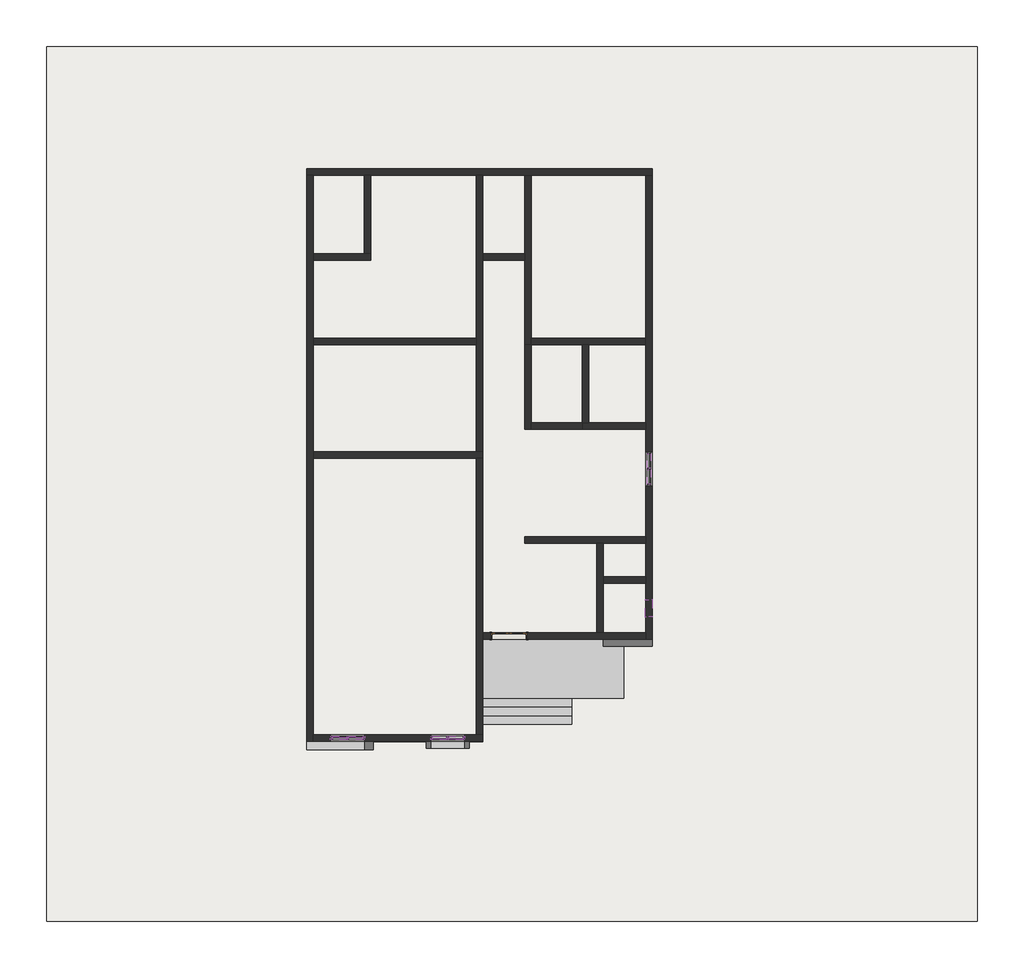
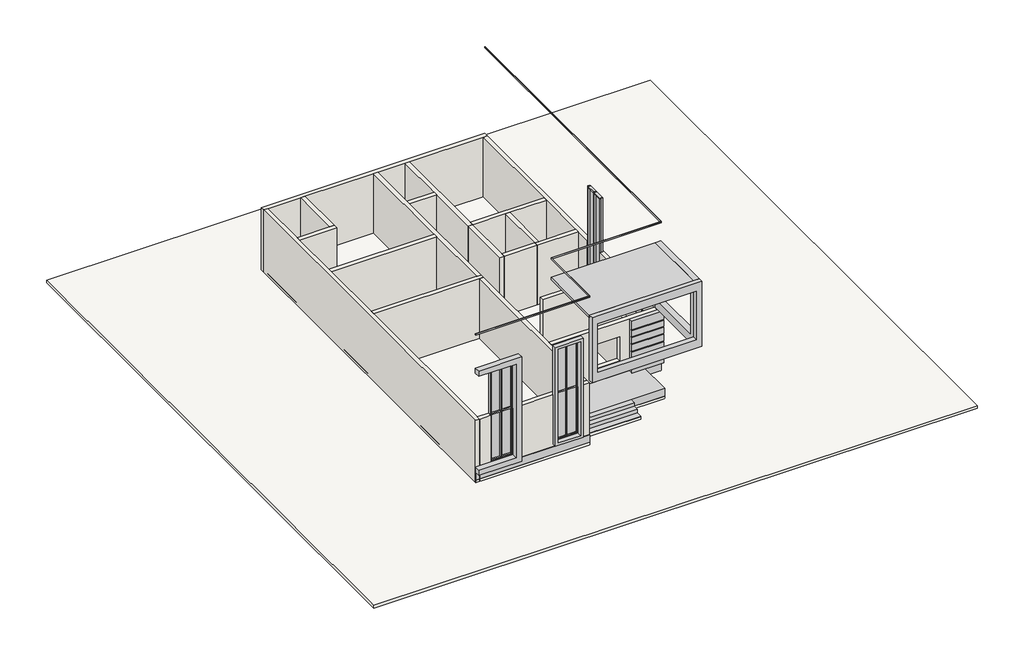
# One storey: 31 members, 21 walls, 10 plates, 2 slabs, 1 door, 1 proxy, 1 window.
"""IFC4 building model written with IfcOpenShell, lengths in millimetres."""

from ifc_helpers import new_model, si_unit, frame, origin, origin_with_axes, place, context, project, spatial, polyline, outline, extrude, faceted_brep, transform, mapped, element, save
from components import door_interior_double_full_glass_wood_4_x_8_0c92ad92, member_25b70949, member_0b7646a3, member_1bc55d26, member_aaa03826, member_6fd72b92, member_6e18fad8, system_panel_glazed_3ff1fc73, system_panel_glazed_5e2fd105, window_f2d8fef0

model = new_model("IFC4")

# Units and contexts
model_context = context("Model", 3, world=origin())
ifc_project = project(units=[si_unit("LENGTHUNIT", "METRE", prefix="MILLI")], contexts=[model_context])

# Site, building, storey
site = spatial("IfcSite", under=ifc_project)
building = spatial("IfcBuilding", under=site)
storey = spatial("IfcBuildingStorey", under=building, Elevation=0.0)

# Proxy
placement = place(None, origin())
element("IfcBuildingElementProxy", 1, Name="Generic Models 1 : Generic Models 1", ObjectType="Generic Models 1 : Generic Models 1", at=placement, inside=storey, context=model_context, shape_type="SweptSolid", body=[
    extrude(outline(polyline([(6324.1896655, -4293.8536251), (914.4, -4293.8536251), (914.4, -6341.6536251), (609.6, -6341.6536251), (609.6, -3989.0536251), (6628.9896655, -3989.0536251), (6628.9896655, -6341.6536251), (6324.1896655, -6341.6536251), (6324.1896655, -4293.8536251)])), frame((0.0, -10008.373087, 0.0), z_axis=(0.0, 1.0, 0.0), x_axis=(0.0, 0.0, 1.0)), (0.0, 0.0, 1.0), 304.8),
    extrude(outline(polyline([(6476.5896655, -585.6536251), (6476.5896655, -2109.6536251), (762.0, -2109.6536251), (762.0, -585.6536251), (6476.5896655, -585.6536251)]), holes=[polyline([(6324.1896655, -738.0536251), (914.4, -738.0536251), (914.4, -1957.2536251), (6324.1896655, -1957.2536251), (6324.1896655, -738.0536251)])]), frame((0.0, -9953.573087, 0.0), z_axis=(0.0, 1.0, 0.0), x_axis=(0.0, 0.0, 1.0)), (0.0, 0.0, 1.0), 250.0),
    extrude(outline(polyline([(-6077.173087, 3597.6), (-6077.173087, 600.0), (-6327.173087, 600.0), (-6327.173087, 922.9293861), (-6276.373087, 922.9293861), (-6276.373087, 975.3927898), (-6327.173087, 975.3927898), (-6327.173087, 1382.9293861), (-6276.373087, 1382.9293861), (-6276.373087, 1435.3927898), (-6327.173087, 1435.3927898), (-6327.173087, 1822.9293861), (-6276.373087, 1822.9293861), (-6276.373087, 1875.3927898), (-6327.173087, 1875.3927898), (-6327.173087, 2242.9293861), (-6276.373087, 2242.9293861), (-6276.373087, 2295.3927898), (-6327.173087, 2295.3927898), (-6327.173087, 2642.9293861), (-6276.373087, 2642.9293861), (-6276.373087, 2695.3927898), (-6327.173087, 2695.3927898), (-6327.173087, 3062.9293861), (-6276.373087, 3062.9293861), (-6276.373087, 3115.3927898), (-6327.173087, 3115.3927898), (-6327.173087, 3597.6), (-6077.173087, 3597.6)])), frame((4169.1463749, 0.0, 0.0), z_axis=(1.0, 0.0, 0.0), x_axis=(0.0, 1.0, 0.0)), (0.0, 0.0, 1.0), 1728.6),
    extrude(outline(polyline([(7500.0, 5897.7463749), (7500.0, -109.4536251), (3750.0, -109.4536251), (3750.0, 5897.7463749), (7500.0, 5897.7463749)]), holes=[polyline([(7042.411304, 5592.9463749), (4243.4748132, 5592.9463749), (4243.4748132, 195.3463749), (7042.411304, 195.3463749), (7042.411304, 5592.9463749)])]), frame((0.0, -9953.573087, 0.0), z_axis=(0.0, 1.0, 0.0), x_axis=(0.0, 0.0, 1.0)), (0.0, 0.0, 1.0), 250.0),
    extrude(outline(polyline([(-9703.573087, 3750.0), (-9703.573087, 7500.0), (-6077.173087, 7500.0), (-6077.173087, 3750.0), (-9703.573087, 3750.0)]), holes=[polyline([(-9398.773087, 4243.4748132), (-6381.973087, 4243.4748132), (-6381.973087, 7042.411304), (-9398.773087, 7042.411304), (-9398.773087, 4243.4748132)])]), frame((5592.9463749, 0.0, 0.0), z_axis=(1.0, 0.0, 0.0), x_axis=(0.0, 1.0, 0.0)), (0.0, 0.0, 1.0), 304.8),
    extrude(outline(polyline([(-109.4536251, -6077.173087), (5592.9463749, -6077.173087), (5592.9463749, -9703.573087), (-109.4536251, -9703.573087), (-109.4536251, -6077.173087)])), frame((0.0, 0.0, 7347.6), z_axis=(0.0, 0.0, 1.0), x_axis=(1.0, 0.0, 0.0)), (0.0, 0.0, 1.0), 152.4),
    extrude(outline(polyline([(4887.2896188, -6077.173087), (4887.2896188, -8177.7312223), (-109.4536251, -8177.7312223), (-109.4536251, -6077.173087), (4887.2896188, -6077.173087)])), origin_with_axes(), (0.0, 0.0, 1.0), 600.0),
    extrude(outline(polyline([(-8177.7312223, 600.0), (-8177.7312223, 0.0), (-9092.1312223, 0.0), (-9092.1312223, 193.6), (-8787.3312223, 193.6), (-8787.3312223, 396.8), (-8482.5312223, 396.8), (-8482.5312223, 600.0), (-8177.7312223, 600.0)])), frame((-109.4536251, 0.0, 0.0), z_axis=(1.0, 0.0, 0.0), x_axis=(0.0, 1.0, 0.0)), (0.0, 0.0, 1.0), 3153.8432439),
    extrude(outline(polyline([(5910.4463749, 10590.826913), (5910.4463749, -6077.173087), (5897.7463749, -6077.173087), (5897.7463749, 10590.826913), (5910.4463749, 10590.826913)])), origin_with_axes(), (0.0, 0.0, 1.0), 600.0),
    extrude(outline(polyline([(5897.7463749, -6089.873087), (4887.2896188, -6089.873087), (4887.2896188, -6077.173087), (5897.7463749, -6077.173087), (5897.7463749, -6089.873087)])), origin_with_axes(), (0.0, 0.0, 1.0), 600.0),
    extrude(outline(polyline([(-109.4536251, -9716.273087), (-6341.6536251, -9716.273087), (-6341.6536251, -9703.573087), (-109.4536251, -9703.573087), (-109.4536251, -9716.273087)])), origin_with_axes(), (0.0, 0.0, 1.0), 609.6),
    extrude(outline(polyline([(-109.4536251, -9716.273087), (-6341.6536251, -9716.273087), (-6341.6536251, -9703.573087), (-109.4536251, -9703.573087), (-109.4536251, -9716.273087)])), frame((0.0, 0.0, 8538.2), z_axis=(0.0, 0.0, 1.0), x_axis=(1.0, 0.0, 0.0)), (0.0, 0.0, 1.0), 76.2),
    extrude(outline(polyline([(-96.7536251, -6077.173087), (-96.7536251, -9716.273087), (-109.4536251, -9716.273087), (-109.4536251, -6077.173087), (-96.7536251, -6077.173087)])), frame((0.0, 0.0, 8538.2), z_axis=(0.0, 0.0, 1.0), x_axis=(1.0, 0.0, 0.0)), (0.0, 0.0, 1.0), 76.2),
    extrude(outline(polyline([(5910.4463749, -6089.873087), (-96.7536251, -6089.873087), (-96.7536251, -6077.173087), (5910.4463749, -6077.173087), (5910.4463749, -6089.873087)])), frame((0.0, 0.0, 8538.2), z_axis=(0.0, 0.0, 1.0), x_axis=(1.0, 0.0, 0.0)), (0.0, 0.0, 1.0), 76.2),
    extrude(outline(polyline([(5910.4463749, 10590.826913), (5910.4463749, -6077.173087), (5897.7463749, -6077.173087), (5897.7463749, 10590.826913), (5910.4463749, 10590.826913)])), frame((0.0, 0.0, 8539.4), z_axis=(0.0, 0.0, 1.0), x_axis=(1.0, 0.0, 0.0)), (0.0, 0.0, 1.0), 75.0),
])

# Door
door_interior_double_full_glass_wood_4_x_8_shape = door_interior_double_full_glass_wood_4_x_8_0c92ad92(model_context)
element("IfcDoor", 2, ObjectType="Door-Interior-Double-Full Glass-Wood : 4' x 8'", at=placement, inside=storey, context=model_context, shape_type="MappedRepresentation", body=[
    mapped(door_interior_double_full_glass_wood_4_x_8_shape, transform((825.5463749, -5959.698087, 609.6), x_axis=(1.0, 0.0, 0.0), y_axis=(0.0, 1.0, 0.0), z_axis=(0.0, 0.0, 1.0))),
])

# Members
member_shape = member_25b70949(model_context)
element("IfcMember", 3, ObjectType="Rectangular Mullion : 2.5\" x 5\" rectangular", at=placement, inside=storey, context=model_context, shape_type="MappedRepresentation", body=[
    mapped(member_shape, transform((-5513.0536251, -9589.273087, 6324.1896655), x_axis=(-1.0, 0.0, 0.0), y_axis=(0.0, -1.0, 0.0), z_axis=(0.0, 0.0, 1.0))),
])
element("IfcMember", 4, ObjectType="Rectangular Mullion : 2.5\" x 5\" rectangular", at=placement, inside=storey, context=model_context, shape_type="MappedRepresentation", body=[
    mapped(member_shape, transform((-738.0536251, -9589.273087, 6324.1896655), x_axis=(1.0, 0.0, 0.0), y_axis=(0.0, 1.0, 0.0), z_axis=(0.0, 0.0, 1.0))),
])
member_2_shape = member_0b7646a3(model_context)
element("IfcMember", 5, ObjectType="Rectangular Mullion : 2.5\" x 5\" rectangular", at=placement, inside=storey, context=model_context, shape_type="MappedRepresentation", body=[
    mapped(member_2_shape, transform((-4357.3536251, -9589.273087, 6324.1896655), x_axis=(0.0, 0.0, 1.0), y_axis=(0.0, -1.0, 0.0), z_axis=(1.0, 0.0, 0.0))),
])
element("IfcMember", 6, ObjectType="Rectangular Mullion : 2.5\" x 5\" rectangular", at=placement, inside=storey, context=model_context, shape_type="MappedRepresentation", body=[
    mapped(member_2_shape, transform((-4935.2036251, -9589.273087, 6324.1896655), x_axis=(0.0, 0.0, 1.0), y_axis=(0.0, -1.0, 0.0), z_axis=(1.0, 0.0, 0.0))),
])
element("IfcMember", 7, ObjectType="Rectangular Mullion : 2.5\" x 5\" rectangular", at=placement, inside=storey, context=model_context, shape_type="MappedRepresentation", body=[
    mapped(member_2_shape, transform((-1893.7536251, -9589.273087, 6324.1896655), x_axis=(0.0, 0.0, 1.0), y_axis=(0.0, 1.0, 0.0), z_axis=(-1.0, 0.0, 0.0))),
])
element("IfcMember", 8, ObjectType="Rectangular Mullion : 2.5\" x 5\" rectangular", at=placement, inside=storey, context=model_context, shape_type="MappedRepresentation", body=[
    mapped(member_2_shape, transform((-1315.9036251, -9589.273087, 6324.1896655), x_axis=(0.0, 0.0, 1.0), y_axis=(0.0, 1.0, 0.0), z_axis=(-1.0, 0.0, 0.0))),
])
element("IfcMember", 9, ObjectType="Rectangular Mullion : 2.5\" x 5\" rectangular", at=placement, inside=storey, context=model_context, shape_type="MappedRepresentation", body=[
    mapped(member_2_shape, transform((5783.4463749, -597.073087, 6707.7288504), x_axis=(0.0, 0.0, 1.0), y_axis=(-1.0, 0.0, 0.0), z_axis=(0.0, -1.0, 0.0))),
])
element("IfcMember", 10, ObjectType="Rectangular Mullion : 2.5\" x 5\" rectangular", at=placement, inside=storey, context=model_context, shape_type="MappedRepresentation", body=[
    mapped(member_2_shape, transform((5783.4463749, -19.223087, 6707.7288504), x_axis=(0.0, 0.0, 1.0), y_axis=(-1.0, 0.0, 0.0), z_axis=(0.0, -1.0, 0.0))),
])
element("IfcMember", 11, ObjectType="Rectangular Mullion : 2.5\" x 5\" rectangular", at=placement, inside=storey, context=model_context, shape_type="MappedRepresentation", body=[
    mapped(member_shape, transform((-4293.8536251, -9589.273087, 914.4), x_axis=(1.0, 0.0, 0.0), y_axis=(0.0, -1.0, 0.0), z_axis=(0.0, 0.0, -1.0))),
])
element("IfcMember", 12, ObjectType="Rectangular Mullion : 2.5\" x 5\" rectangular", at=placement, inside=storey, context=model_context, shape_type="MappedRepresentation", body=[
    mapped(member_shape, transform((-1957.2536251, -9589.273087, 914.4), x_axis=(-1.0, 0.0, 0.0), y_axis=(0.0, 1.0, 0.0), z_axis=(0.0, 0.0, -1.0))),
])
element("IfcMember", 13, ObjectType="Rectangular Mullion : 2.5\" x 5\" rectangular", at=placement, inside=storey, context=model_context, shape_type="MappedRepresentation", body=[
    mapped(member_2_shape, transform((-5449.5536251, -9589.273087, 914.4), x_axis=(0.0, 0.0, -1.0), y_axis=(0.0, -1.0, 0.0), z_axis=(-1.0, 0.0, 0.0))),
])
element("IfcMember", 14, ObjectType="Rectangular Mullion : 2.5\" x 5\" rectangular", at=placement, inside=storey, context=model_context, shape_type="MappedRepresentation", body=[
    mapped(member_2_shape, transform((-4871.7036251, -9589.273087, 914.4), x_axis=(0.0, 0.0, -1.0), y_axis=(0.0, -1.0, 0.0), z_axis=(-1.0, 0.0, 0.0))),
])
element("IfcMember", 15, ObjectType="Rectangular Mullion : 2.5\" x 5\" rectangular", at=placement, inside=storey, context=model_context, shape_type="MappedRepresentation", body=[
    mapped(member_2_shape, transform((-801.5536251, -9589.273087, 914.4), x_axis=(0.0, 0.0, -1.0), y_axis=(0.0, 1.0, 0.0), z_axis=(1.0, 0.0, 0.0))),
])
element("IfcMember", 16, ObjectType="Rectangular Mullion : 2.5\" x 5\" rectangular", at=placement, inside=storey, context=model_context, shape_type="MappedRepresentation", body=[
    mapped(member_2_shape, transform((-1379.4036251, -9589.273087, 914.4), x_axis=(0.0, 0.0, -1.0), y_axis=(0.0, 1.0, 0.0), z_axis=(1.0, 0.0, 0.0))),
])
element("IfcMember", 17, ObjectType="Rectangular Mullion : 2.5\" x 5\" rectangular", at=placement, inside=storey, context=model_context, shape_type="MappedRepresentation", body=[
    mapped(member_2_shape, transform((5783.4463749, 495.126913, 914.4), x_axis=(0.0, 0.0, -1.0), y_axis=(-1.0, 0.0, 0.0), z_axis=(0.0, 1.0, 0.0))),
])
element("IfcMember", 18, ObjectType="Rectangular Mullion : 2.5\" x 5\" rectangular", at=placement, inside=storey, context=model_context, shape_type="MappedRepresentation", body=[
    mapped(member_2_shape, transform((5783.4463749, -82.723087, 914.4), x_axis=(0.0, 0.0, -1.0), y_axis=(-1.0, 0.0, 0.0), z_axis=(0.0, 1.0, 0.0))),
])
member_3_shape = member_1bc55d26(model_context)
element("IfcMember", 19, ObjectType="Rectangular Mullion : 2.5\" x 5\" rectangular", at=placement, inside=storey, context=model_context, shape_type="MappedRepresentation", body=[
    mapped(member_3_shape, transform((-4903.4536251, -9589.273087, 914.4), x_axis=(1.0, 0.0, 0.0), y_axis=(0.0, -1.0, 0.0), z_axis=(0.0, 0.0, -1.0))),
])
element("IfcMember", 20, ObjectType="Rectangular Mullion : 2.5\" x 5\" rectangular", at=placement, inside=storey, context=model_context, shape_type="MappedRepresentation", body=[
    mapped(member_3_shape, transform((-1347.6536251, -9589.273087, 914.4), x_axis=(-1.0, 0.0, 0.0), y_axis=(0.0, 1.0, 0.0), z_axis=(0.0, 0.0, -1.0))),
])
member_4_shape = member_aaa03826(model_context)
element("IfcMember", 21, ObjectType="Rectangular Mullion : 2.5\" x 5\" rectangular", at=placement, inside=storey, context=model_context, shape_type="MappedRepresentation", body=[
    mapped(member_4_shape, transform((-4935.2036251, -9589.273087, 3619.2948327), x_axis=(0.0, 0.0, 1.0), y_axis=(0.0, -1.0, 0.0), z_axis=(1.0, 0.0, 0.0))),
])
element("IfcMember", 22, ObjectType="Rectangular Mullion : 2.5\" x 5\" rectangular", at=placement, inside=storey, context=model_context, shape_type="MappedRepresentation", body=[
    mapped(member_4_shape, transform((-4357.3536251, -9589.273087, 3619.2948327), x_axis=(0.0, 0.0, 1.0), y_axis=(0.0, -1.0, 0.0), z_axis=(1.0, 0.0, 0.0))),
])
element("IfcMember", 23, ObjectType="Rectangular Mullion : 2.5\" x 5\" rectangular", at=placement, inside=storey, context=model_context, shape_type="MappedRepresentation", body=[
    mapped(member_4_shape, transform((-1315.9036251, -9589.273087, 3619.2948327), x_axis=(0.0, 0.0, 1.0), y_axis=(0.0, 1.0, 0.0), z_axis=(-1.0, 0.0, 0.0))),
])
element("IfcMember", 24, ObjectType="Rectangular Mullion : 2.5\" x 5\" rectangular", at=placement, inside=storey, context=model_context, shape_type="MappedRepresentation", body=[
    mapped(member_4_shape, transform((-1893.7536251, -9589.273087, 3619.2948327), x_axis=(0.0, 0.0, 1.0), y_axis=(0.0, 1.0, 0.0), z_axis=(-1.0, 0.0, 0.0))),
])
element("IfcMember", 25, ObjectType="Rectangular Mullion : 2.5\" x 5\" rectangular", at=placement, inside=storey, context=model_context, shape_type="MappedRepresentation", body=[
    mapped(member_shape, transform((-4293.8536251, -9589.273087, 3619.2948327), x_axis=(1.0, 0.0, 0.0), y_axis=(0.0, -1.0, 0.0), z_axis=(0.0, 0.0, -1.0))),
])
element("IfcMember", 26, ObjectType="Rectangular Mullion : 2.5\" x 5\" rectangular", at=placement, inside=storey, context=model_context, shape_type="MappedRepresentation", body=[
    mapped(member_shape, transform((-1957.2536251, -9589.273087, 3619.2948327), x_axis=(-1.0, 0.0, 0.0), y_axis=(0.0, 1.0, 0.0), z_axis=(0.0, 0.0, -1.0))),
])
element("IfcMember", 27, ObjectType="Rectangular Mullion : 2.5\" x 5\" rectangular", at=placement, inside=storey, context=model_context, shape_type="MappedRepresentation", body=[
    mapped(member_shape, transform((-5513.0536251, -9589.273087, 3619.2948327), x_axis=(-1.0, 0.0, 0.0), y_axis=(0.0, -1.0, 0.0), z_axis=(0.0, 0.0, 1.0))),
])
element("IfcMember", 28, ObjectType="Rectangular Mullion : 2.5\" x 5\" rectangular", at=placement, inside=storey, context=model_context, shape_type="MappedRepresentation", body=[
    mapped(member_shape, transform((-738.0536251, -9589.273087, 3619.2948327), x_axis=(1.0, 0.0, 0.0), y_axis=(0.0, 1.0, 0.0), z_axis=(0.0, 0.0, 1.0))),
])
element("IfcMember", 29, ObjectType="Rectangular Mullion : 2.5\" x 5\" rectangular", at=placement, inside=storey, context=model_context, shape_type="MappedRepresentation", body=[
    mapped(member_3_shape, transform((-4903.4536251, -9589.273087, 3619.2948327), x_axis=(1.0, 0.0, 0.0), y_axis=(0.0, -1.0, 0.0), z_axis=(0.0, 0.0, -1.0))),
])
element("IfcMember", 30, ObjectType="Rectangular Mullion : 2.5\" x 5\" rectangular", at=placement, inside=storey, context=model_context, shape_type="MappedRepresentation", body=[
    mapped(member_3_shape, transform((-1347.6536251, -9589.273087, 3619.2948327), x_axis=(-1.0, 0.0, 0.0), y_axis=(0.0, 1.0, 0.0), z_axis=(0.0, 0.0, -1.0))),
])
member_5_shape = member_6fd72b92(model_context)
element("IfcMember", 31, ObjectType="Rectangular Mullion : 2.5\" x 5\" rectangular", at=placement, inside=storey, context=model_context, shape_type="MappedRepresentation", body=[
    mapped(member_5_shape, transform((5783.4463749, -50.973087, 914.4), x_axis=(0.0, -1.0, 0.0), y_axis=(-1.0, 0.0, 0.0), z_axis=(0.0, 0.0, -1.0))),
])
member_6_shape = member_6e18fad8(model_context)
element("IfcMember", 32, ObjectType="Rectangular Mullion : 2.5\" x 5\" rectangular", at=placement, inside=storey, context=model_context, shape_type="MappedRepresentation", body=[
    mapped(member_6_shape, transform((5783.4463749, 558.626913, 6707.7288504), x_axis=(0.0, 1.0, 0.0), y_axis=(-1.0, 0.0, 0.0), z_axis=(0.0, 0.0, 1.0))),
])
element("IfcMember", 33, ObjectType="Rectangular Mullion : 2.5\" x 5\" rectangular", at=placement, inside=storey, context=model_context, shape_type="MappedRepresentation", body=[
    mapped(member_6_shape, transform((5783.4463749, -660.573087, 914.4), x_axis=(0.0, -1.0, 0.0), y_axis=(-1.0, 0.0, 0.0), z_axis=(0.0, 0.0, -1.0))),
])

# Plates
element("IfcPlate", 34, ObjectType="System Panel : Glazed", at=placement, inside=storey, context=model_context, shape_type="SweptSolid", body=[
    extrude(outline(polyline([(-4935.2036251, -9570.223087), (-5449.5536251, -9570.223087), (-5449.5536251, -9544.823087), (-4935.2036251, -9544.823087), (-4935.2036251, -9570.223087)])), frame((0.0, 0.0, 977.9), z_axis=(0.0, 0.0, 1.0), x_axis=(1.0, 0.0, 0.0)), (0.0, 0.0, 1.0), 2609.6448327),
])
element("IfcPlate", 35, ObjectType="System Panel : Glazed", at=placement, inside=storey, context=model_context, shape_type="SweptSolid", body=[
    extrude(outline(polyline([(5802.4963749, -19.223087), (5802.4963749, 495.126913), (5827.8963749, 495.126913), (5827.8963749, -19.223087), (5802.4963749, -19.223087)])), frame((0.0, 0.0, 977.9), z_axis=(0.0, 0.0, 1.0), x_axis=(1.0, 0.0, 0.0)), (0.0, 0.0, 1.0), 5666.3288504),
])
system_panel_glazed_shape = system_panel_glazed_3ff1fc73(model_context)
element("IfcPlate", 36, ObjectType="System Panel : Glazed", at=placement, inside=storey, context=model_context, shape_type="MappedRepresentation", body=[
    mapped(system_panel_glazed_shape, transform((-1058.7286251, -9589.273087, 977.9), x_axis=(-1.0, 0.0, 0.0), y_axis=(0.0, -1.0, 0.0), z_axis=(0.0, 0.0, 1.0))),
])
element("IfcPlate", 37, ObjectType="System Panel : Glazed", at=placement, inside=storey, context=model_context, shape_type="MappedRepresentation", body=[
    mapped(system_panel_glazed_shape, transform((-4614.5286251, -9589.273087, 977.9), x_axis=(1.0, 0.0, 0.0), y_axis=(0.0, 1.0, 0.0), z_axis=(0.0, 0.0, 1.0))),
])
element("IfcPlate", 38, ObjectType="System Panel : Glazed", at=placement, inside=storey, context=model_context, shape_type="MappedRepresentation", body=[
    mapped(system_panel_glazed_shape, transform((-1636.5786251, -9589.273087, 977.9), x_axis=(-1.0, 0.0, 0.0), y_axis=(0.0, -1.0, 0.0), z_axis=(0.0, 0.0, 1.0))),
])
element("IfcPlate", 39, ObjectType="System Panel : Glazed", at=placement, inside=storey, context=model_context, shape_type="MappedRepresentation", body=[
    mapped(system_panel_glazed_shape, transform((-5192.3786251, -9589.273087, 3651.0448327), x_axis=(1.0, 0.0, 0.0), y_axis=(0.0, 1.0, 0.0), z_axis=(0.0, 0.0, 1.0))),
])
element("IfcPlate", 40, ObjectType="System Panel : Glazed", at=placement, inside=storey, context=model_context, shape_type="MappedRepresentation", body=[
    mapped(system_panel_glazed_shape, transform((-4614.5286251, -9589.273087, 3651.0448327), x_axis=(1.0, 0.0, 0.0), y_axis=(0.0, 1.0, 0.0), z_axis=(0.0, 0.0, 1.0))),
])
element("IfcPlate", 41, ObjectType="System Panel : Glazed", at=placement, inside=storey, context=model_context, shape_type="MappedRepresentation", body=[
    mapped(system_panel_glazed_shape, transform((-1058.7286251, -9589.273087, 3651.0448327), x_axis=(-1.0, 0.0, 0.0), y_axis=(0.0, -1.0, 0.0), z_axis=(0.0, 0.0, 1.0))),
])
element("IfcPlate", 42, ObjectType="System Panel : Glazed", at=placement, inside=storey, context=model_context, shape_type="MappedRepresentation", body=[
    mapped(system_panel_glazed_shape, transform((-1636.5786251, -9589.273087, 3651.0448327), x_axis=(-1.0, 0.0, 0.0), y_axis=(0.0, -1.0, 0.0), z_axis=(0.0, 0.0, 1.0))),
])
system_panel_glazed_2_shape = system_panel_glazed_5e2fd105(model_context)
element("IfcPlate", 43, ObjectType="System Panel : Glazed", at=placement, inside=storey, context=model_context, shape_type="MappedRepresentation", body=[
    mapped(system_panel_glazed_2_shape, transform((5783.4463749, -339.898087, 977.9), x_axis=(0.0, -1.0, 0.0), y_axis=(1.0, 0.0, 0.0), z_axis=(0.0, 0.0, 1.0))),
])

# Slabs
element("IfcSlab", 44, ObjectType="6\" floor gf", at=placement, inside=storey, context=model_context, shape_type="SweptSolid", body=[
    extrude(outline(polyline([(-6341.6536251, 10590.826913), (5910.4463749, 10590.826913), (5910.4463749, -6077.173087), (4887.2896188, -6077.173087), (4887.2896188, -8177.7312223), (3044.3896188, -8177.7312223), (3044.3896188, -9092.1312223), (-109.4536251, -9092.1312223), (-109.4536251, -9716.273087), (-6341.6536251, -9716.273087), (-6341.6536251, 10590.826913)])), frame((0.0, 0.0, 0.1), z_axis=(0.0, 0.0, 1.0), x_axis=(1.0, 0.0, 0.0)), (0.0, 0.0, 1.0), 152.4),
])
element("IfcSlab", 45, ObjectType="6\" floor site", at=placement, inside=storey, context=model_context, shape_type="SweptSolid", body=[
    extrude(outline(polyline([(17430.7723404, 14927.3285807), (17430.7723404, -16072.6714193), (-15569.2276596, -16072.6714193), (-15569.2276596, 14927.3285807), (17430.7723404, 14927.3285807)])), frame((0.0, 0.0, -152.4), z_axis=(0.0, 0.0, 1.0), x_axis=(1.0, 0.0, 0.0)), (0.0, 0.0, 1.0), 152.4),
])

# Walls
element("IfcWall", 46, ObjectType="9\" wall", at=placement, inside=storey, context=model_context, shape_type="Brep", body=[
    faceted_brep([(-6341.6536251, 10362.226913, 0.0), (-6113.0536251, 10362.226913, 0.0), (-4313.0536251, 10362.226913, 0.0), (-4084.4536251, 10362.226913, 0.0), (-338.0536251, 10362.226913, 0.0), (-109.4536251, 10362.226913, 0.0), (1390.5463749, 10362.226913, 0.0), (1619.1463749, 10362.226913, 0.0), (5669.1463749, 10362.226913, 0.0), (5897.7463749, 10362.226913, 0.0), (5897.7463749, 10362.226913, 3597.6), (5669.1463749, 10362.226913, 3597.6), (1619.1463749, 10362.226913, 3597.6), (1390.5463749, 10362.226913, 3597.6), (-109.4536251, 10362.226913, 3597.6), (-338.0536251, 10362.226913, 3597.6), (-4084.4536251, 10362.226913, 3597.6), (-4313.0536251, 10362.226913, 3597.6), (-6113.0536251, 10362.226913, 3597.6), (-6341.6536251, 10362.226913, 3597.6), (-6341.6536251, 10590.826913, 0.0), (-6341.6536251, 10590.826913, 3597.6), (5897.7463749, 10590.826913, 3597.6), (5897.7463749, 10590.826913, 0.0)], [[[0, 1, 2, 3, 4, 5, 6, 7, 8, 9, 10, 11, 12, 13, 14, 15, 16, 17, 18, 19]], [[20, 21, 22, 23]], [[9, 8, 7, 6, 5, 4, 3, 2, 1, 0, 20, 23]], [[0, 19, 21, 20]], [[10, 9, 23, 22]], [[19, 18, 17, 16, 15, 14, 13, 12, 11, 10, 22, 21]]]),
])
element("IfcWall", 47, ObjectType="9\" wall", at=placement, inside=storey, context=model_context, shape_type="Brep", body=[
    faceted_brep([(-6113.0536251, -9703.573087, 0.0), (-6113.0536251, -9474.973087, 0.0), (-6113.0536251, 330.026913, 0.0), (-6113.0536251, 558.626913, 0.0), (-6113.0536251, 4358.626913, 0.0), (-6113.0536251, 4587.226913, 0.0), (-6113.0536251, 7358.626913, 0.0), (-6113.0536251, 7587.226913, 0.0), (-6113.0536251, 10362.226913, 0.0), (-6113.0536251, 10362.226913, 3597.6), (-6113.0536251, 7587.226913, 3597.6), (-6113.0536251, 7358.626913, 3597.6), (-6113.0536251, 4587.226913, 3597.6), (-6113.0536251, 4358.626913, 3597.6), (-6113.0536251, 558.626913, 3597.6), (-6113.0536251, 330.026913, 3597.6), (-6113.0536251, -9474.973087, 3597.6), (-6113.0536251, -9703.573087, 3597.6), (-6341.6536251, -9703.573087, 0.0), (-6341.6536251, -9703.573087, 3597.6), (-6341.6536251, 10362.226913, 3597.6), (-6341.6536251, 10362.226913, 0.0)], [[[0, 1, 2, 3, 4, 5, 6, 7, 8, 9, 10, 11, 12, 13, 14, 15, 16, 17]], [[18, 19, 20, 21]], [[8, 7, 6, 5, 4, 3, 2, 1, 0, 18, 21]], [[9, 8, 21, 20]], [[0, 17, 19, 18]], [[17, 16, 15, 14, 13, 12, 11, 10, 9, 20, 19]]]),
])
element("IfcWall", 48, ObjectType="9\" wall", at=placement, inside=storey, context=model_context, shape_type="Brep", body=[
    faceted_brep([(-6113.0536251, 7358.626913, 0.0), (-4084.4536251, 7358.626913, 0.0), (-4084.4536251, 7358.626913, 3597.6), (-6113.0536251, 7358.626913, 3597.6), (-6113.0536251, 7587.226913, 0.0), (-6113.0536251, 7587.226913, 3597.6), (-4313.0536251, 7587.226913, 3597.6), (-4084.4536251, 7587.226913, 3597.6), (-4084.4536251, 7587.226913, 0.0), (-4313.0536251, 7587.226913, 0.0)], [[[0, 1, 2, 3]], [[4, 5, 6, 7, 8, 9]], [[1, 0, 4, 9, 8]], [[0, 3, 5, 4]], [[2, 1, 8, 7]], [[3, 2, 7, 6, 5]]]),
])
element("IfcWall", 49, ObjectType="9\" wall", at=placement, inside=storey, context=model_context, shape_type="SweptSolid", body=[
    extrude(outline(polyline([(-4084.4536251, 10362.226913), (-4084.4536251, 7587.226913), (-4313.0536251, 7587.226913), (-4313.0536251, 10362.226913), (-4084.4536251, 10362.226913)])), origin_with_axes(), (0.0, 0.0, 1.0), 3597.6),
])
element("IfcWall", 50, ObjectType="9\" wall", at=placement, inside=storey, context=model_context, shape_type="SweptSolid", body=[
    extrude(outline(polyline([(-338.0536251, 4358.626913), (-6113.0536251, 4358.626913), (-6113.0536251, 4587.226913), (-338.0536251, 4587.226913), (-338.0536251, 4358.626913)])), origin_with_axes(), (0.0, 0.0, 1.0), 3597.6),
])
element("IfcWall", 51, ObjectType="9\" wall", at=placement, inside=storey, context=model_context, shape_type="Brep", body=[
    faceted_brep([(-109.4536251, 558.626913, 0.0), (-109.4536251, 7358.626913, 0.0), (-109.4536251, 7587.226913, 0.0), (-109.4536251, 10362.226913, 0.0), (-109.4536251, 10362.226913, 3597.6), (-109.4536251, 7587.226913, 3597.6), (-109.4536251, 7358.626913, 3597.6), (-109.4536251, 558.626913, 3597.6), (-338.0536251, 558.626913, 0.0), (-338.0536251, 558.626913, 3597.6), (-338.0536251, 4358.626913, 3597.6), (-338.0536251, 4587.226913, 3597.6), (-338.0536251, 10362.226913, 3597.6), (-338.0536251, 10362.226913, 0.0), (-338.0536251, 4587.226913, 0.0), (-338.0536251, 4358.626913, 0.0)], [[[0, 1, 2, 3, 4, 5, 6, 7]], [[8, 9, 10, 11, 12, 13, 14, 15]], [[3, 2, 1, 0, 8, 15, 14, 13]], [[4, 3, 13, 12]], [[0, 7, 9, 8]], [[7, 6, 5, 4, 12, 11, 10, 9]]]),
])
element("IfcWall", 52, ObjectType="9\" wall", at=placement, inside=storey, context=model_context, shape_type="Brep", body=[
    faceted_brep([(-6113.0536251, 330.026913, 0.0), (-338.0536251, 330.026913, 0.0), (-109.4536251, 330.026913, 0.0), (-109.4536251, 330.026913, 3597.6), (-338.0536251, 330.026913, 3597.6), (-6113.0536251, 330.026913, 3597.6), (-6113.0536251, 558.626913, 0.0), (-6113.0536251, 558.626913, 3597.6), (-338.0536251, 558.626913, 3597.6), (-109.4536251, 558.626913, 3597.6), (-109.4536251, 558.626913, 0.0), (-338.0536251, 558.626913, 0.0)], [[[0, 1, 2, 3, 4, 5]], [[6, 7, 8, 9, 10, 11]], [[2, 1, 0, 6, 11, 10]], [[0, 5, 7, 6]], [[3, 2, 10, 9]], [[5, 4, 3, 9, 8, 7]]]),
])
element("IfcWall", 53, ObjectType="9\" wall", at=placement, inside=storey, context=model_context, shape_type="Brep", body=[
    faceted_brep([(-6113.0536251, -9703.573087, 0.0), (-109.4536251, -9703.573087, 0.0), (-109.4536251, -9703.573087, 3597.6), (-738.0536251, -9703.573087, 3597.6), (-738.0536251, -9703.573087, 914.4), (-1957.2536251, -9703.573087, 914.4), (-1957.2536251, -9703.573087, 3597.6), (-4293.8536251, -9703.573087, 3597.6), (-4293.8536251, -9703.573087, 914.4), (-5513.0536251, -9703.573087, 914.4), (-5513.0536251, -9703.573087, 3597.6), (-6113.0536251, -9703.573087, 3597.6), (-109.4536251, -9474.973087, 0.0), (-338.0536251, -9474.973087, 0.0), (-6113.0536251, -9474.973087, 0.0), (-6113.0536251, -9474.973087, 3597.6), (-5513.0536251, -9474.973087, 3597.6), (-5513.0536251, -9474.973087, 914.4), (-4293.8536251, -9474.973087, 914.4), (-4293.8536251, -9474.973087, 3597.6), (-1957.2536251, -9474.973087, 3597.6), (-1957.2536251, -9474.973087, 914.4), (-738.0536251, -9474.973087, 914.4), (-738.0536251, -9474.973087, 3597.6), (-338.0536251, -9474.973087, 3597.6), (-109.4536251, -9474.973087, 3597.6)], [[[0, 1, 2, 3, 4, 5, 6, 7, 8, 9, 10, 11]], [[12, 13, 14, 15, 16, 17, 18, 19, 20, 21, 22, 23, 24, 25]], [[1, 0, 14, 13, 12]], [[2, 1, 12, 25]], [[0, 11, 15, 14]], [[9, 17, 16, 10]], [[18, 8, 7, 19]], [[17, 9, 8, 18]], [[22, 4, 3, 23]], [[5, 21, 20, 6]], [[4, 22, 21, 5]], [[2, 25, 24, 23, 3]], [[15, 11, 10, 16]], [[19, 7, 6, 20]]]),
])
element("IfcWall", 54, ObjectType="9\" wall", at=placement, inside=storey, context=model_context, shape_type="Brep", body=[
    faceted_brep([(-109.4536251, -9474.973087, 0.0), (-109.4536251, -6077.173087, 0.0), (-109.4536251, -5848.573087, 0.0), (-109.4536251, 330.026913, 0.0), (-109.4536251, 330.026913, 3597.6), (-109.4536251, -5848.573087, 3597.6), (-109.4536251, -6077.173087, 3597.6), (-109.4536251, -9474.973087, 3597.6), (-338.0536251, -9474.973087, 0.0), (-338.0536251, -9474.973087, 3597.6), (-338.0536251, 330.026913, 3597.6), (-338.0536251, 330.026913, 0.0)], [[[0, 1, 2, 3, 4, 5, 6, 7]], [[8, 9, 10, 11]], [[3, 2, 1, 0, 8, 11]], [[0, 7, 9, 8]], [[4, 3, 11, 10]], [[7, 6, 5, 4, 10, 9]]]),
])
element("IfcWall", 55, ObjectType="9\" wall", at=placement, inside=storey, context=model_context, shape_type="Brep", body=[
    faceted_brep([(1390.5463749, 10362.226913, 0.0), (1390.5463749, 7587.226913, 0.0), (1390.5463749, 7358.626913, 0.0), (1390.5463749, 4358.626913, 0.0), (1390.5463749, 4358.626913, 3597.6), (1390.5463749, 7358.626913, 3597.6), (1390.5463749, 7587.226913, 3597.6), (1390.5463749, 10362.226913, 3597.6), (1619.1463749, 10362.226913, 0.0), (1619.1463749, 10362.226913, 3597.6), (1619.1463749, 4587.226913, 3597.6), (1619.1463749, 4358.626913, 3597.6), (1619.1463749, 4358.626913, 0.0), (1619.1463749, 4587.226913, 0.0), (1615.5463749, 4358.626913, 0.0), (1615.5463749, 4358.626913, 3597.6)], [[[0, 1, 2, 3, 4, 5, 6, 7]], [[8, 9, 10, 11, 12, 13]], [[3, 2, 1, 0, 8, 13, 12, 14]], [[0, 7, 9, 8]], [[4, 3, 14, 12, 11, 15]], [[7, 6, 5, 4, 15, 11, 10, 9]]]),
])
element("IfcWall", 56, ObjectType="9\" wall", at=placement, inside=storey, context=model_context, shape_type="SweptSolid", body=[
    extrude(outline(polyline([(-109.4536251, 7587.226913), (1390.5463749, 7587.226913), (1390.5463749, 7358.626913), (-109.4536251, 7358.626913), (-109.4536251, 7587.226913)])), origin_with_axes(), (0.0, 0.0, 1.0), 3597.6),
])
element("IfcWall", 57, ObjectType="9\" wall", at=placement, inside=storey, context=model_context, shape_type="Brep", body=[
    faceted_brep([(5669.1463749, 10362.226913, 0.0), (5669.1463749, 4587.226913, 0.0), (5669.1463749, 4358.626913, 0.0), (5669.1463749, 1583.626913, 0.0), (5669.1463749, 1355.026913, 0.0), (5669.1463749, -2444.973087, 0.0), (5669.1463749, -2673.573087, 0.0), (5669.1463749, -3873.573087, 0.0), (5669.1463749, -4102.173087, 0.0), (5669.1463749, -5848.573087, 0.0), (5669.1463749, -6077.173087, 0.0), (5669.1463749, -6077.173087, 3597.6), (5669.1463749, -5848.573087, 3597.6), (5669.1463749, -4102.173087, 3597.6), (5669.1463749, -3873.573087, 3597.6), (5669.1463749, -2673.573087, 3597.6), (5669.1463749, -2444.973087, 3597.6), (5669.1463749, -660.573087, 3597.6), (5669.1463749, -660.573087, 914.4), (5669.1463749, 558.626913, 914.4), (5669.1463749, 558.626913, 3597.6), (5669.1463749, 1355.026913, 3597.6), (5669.1463749, 1583.626913, 3597.6), (5669.1463749, 4358.626913, 3597.6), (5669.1463749, 4587.226913, 3597.6), (5669.1463749, 10362.226913, 3597.6), (5669.1463749, -4680.098087, 2743.2), (5669.1463749, -5289.698087, 2743.2), (5669.1463749, -5289.698087, 2133.6), (5669.1463749, -4680.098087, 2133.6), (5897.7463749, -6077.173087, 0.0), (5897.7463749, 10362.226913, 0.0), (5897.7463749, 10362.226913, 3597.6), (5897.7463749, 558.626913, 3597.6), (5897.7463749, 558.626913, 914.4), (5897.7463749, -660.573087, 914.4), (5897.7463749, -660.573087, 3597.6), (5897.7463749, -6077.173087, 3597.6), (5897.7463749, -4680.098087, 2743.2), (5897.7463749, -4680.098087, 2133.6), (5897.7463749, -5289.698087, 2133.6), (5897.7463749, -5289.698087, 2743.2)], [[[0, 1, 2, 3, 4, 5, 6, 7, 8, 9, 10, 11, 12, 13, 14, 15, 16, 17, 18, 19, 20, 21, 22, 23, 24, 25], [26, 27, 28, 29]], [[30, 31, 32, 33, 34, 35, 36, 37], [38, 39, 40, 41]], [[10, 9, 8, 7, 6, 5, 4, 3, 2, 1, 0, 31, 30]], [[0, 25, 32, 31]], [[11, 10, 30, 37]], [[11, 37, 36, 17, 16, 15, 14, 13, 12]], [[32, 25, 24, 23, 22, 21, 20, 33]], [[39, 38, 26, 29]], [[40, 39, 29, 28]], [[41, 40, 28, 27]], [[38, 41, 27, 26]], [[19, 34, 33, 20]], [[35, 18, 17, 36]], [[34, 19, 18, 35]]]),
])
element("IfcWall", 58, ObjectType="9\" wall", at=placement, inside=storey, context=model_context, shape_type="Brep", body=[
    faceted_brep([(5669.1463749, 4587.226913, 0.0), (1619.1463749, 4587.226913, 0.0), (1619.1463749, 4587.226913, 3597.6), (5669.1463749, 4587.226913, 3597.6), (5669.1463749, 4358.626913, 0.0), (5669.1463749, 4358.626913, 3597.6), (3644.1463749, 4358.626913, 3597.6), (3415.5463749, 4358.626913, 3597.6), (1619.1463749, 4358.626913, 3597.6), (1619.1463749, 4358.626913, 0.0), (3415.5463749, 4358.626913, 0.0), (3644.1463749, 4358.626913, 0.0)], [[[0, 1, 2, 3]], [[4, 5, 6, 7, 8, 9, 10, 11]], [[1, 0, 4, 11, 10, 9]], [[2, 1, 9, 8]], [[0, 3, 5, 4]], [[3, 2, 8, 7, 6, 5]]]),
])
element("IfcWall", 59, ObjectType="9\" wall", at=placement, inside=storey, context=model_context, shape_type="Brep", body=[
    faceted_brep([(5669.1463749, 1583.626913, 0.0), (3644.1463749, 1583.626913, 0.0), (3415.5463749, 1583.626913, 0.0), (3415.5463749, 1583.626913, 3597.6), (3644.1463749, 1583.626913, 3597.6), (5669.1463749, 1583.626913, 3597.6), (5669.1463749, 1355.026913, 0.0), (5669.1463749, 1355.026913, 3597.6), (3415.5463749, 1355.026913, 3597.6), (3415.5463749, 1355.026913, 0.0)], [[[0, 1, 2, 3, 4, 5]], [[6, 7, 8, 9]], [[2, 1, 0, 6, 9]], [[0, 5, 7, 6]], [[3, 2, 9, 8]], [[5, 4, 3, 8, 7]]]),
])
element("IfcWall", 60, ObjectType="9\" wall", at=placement, inside=storey, context=model_context, shape_type="SweptSolid", body=[
    extrude(outline(polyline([(3644.1463749, 4358.626913), (3644.1463749, 1583.626913), (3415.5463749, 1583.626913), (3415.5463749, 4358.626913), (3644.1463749, 4358.626913)])), origin_with_axes(), (0.0, 0.0, 1.0), 3597.6),
])
element("IfcWall", 61, ObjectType="9\" wall", at=placement, inside=storey, context=model_context, shape_type="Brep", body=[
    faceted_brep([(1386.9463749, 4358.626913, 0.0), (1386.9463749, 1355.026913, 0.0), (1386.9463749, 1355.026913, 3597.6), (1386.9463749, 4358.626913, 3597.6), (1615.5463749, 4358.626913, 0.0), (1615.5463749, 4358.626913, 3597.6), (1615.5463749, 1583.626913, 3597.6), (1615.5463749, 1355.026913, 3597.6), (1615.5463749, 1355.026913, 0.0), (1615.5463749, 1583.626913, 0.0), (1390.5463749, 4358.626913, 0.0), (1390.5463749, 4358.626913, 3597.6)], [[[0, 1, 2, 3]], [[4, 5, 6, 7, 8, 9]], [[1, 0, 10, 4, 9, 8]], [[0, 3, 11, 5, 4, 10]], [[2, 1, 8, 7]], [[3, 2, 7, 6, 5, 11]]]),
])
element("IfcWall", 62, ObjectType="9\" wall", at=placement, inside=storey, context=model_context, shape_type="SweptSolid", body=[
    extrude(outline(polyline([(3415.5463749, 1355.026913), (1615.5463749, 1355.026913), (1615.5463749, 1583.626913), (3415.5463749, 1583.626913), (3415.5463749, 1355.026913)])), origin_with_axes(), (0.0, 0.0, 1.0), 3597.6),
])
element("IfcWall", 63, ObjectType="9\" wall", at=placement, inside=storey, context=model_context, shape_type="Brep", body=[
    faceted_brep([(5669.1463749, -2444.973087, 0.0), (1390.5463749, -2444.973087, 0.0), (1390.5463749, -2444.973087, 3597.6), (5669.1463749, -2444.973087, 3597.6), (5669.1463749, -2673.573087, 0.0), (5669.1463749, -2673.573087, 3597.6), (4169.1463749, -2673.573087, 3597.6), (3940.5463749, -2673.573087, 3597.6), (1390.5463749, -2673.573087, 3597.6), (1390.5463749, -2673.573087, 0.0), (3940.5463749, -2673.573087, 0.0), (4169.1463749, -2673.573087, 0.0)], [[[0, 1, 2, 3]], [[4, 5, 6, 7, 8, 9, 10, 11]], [[1, 0, 4, 11, 10, 9]], [[2, 1, 9, 8]], [[0, 3, 5, 4]], [[3, 2, 8, 7, 6, 5]]]),
])
element("IfcWall", 64, ObjectType="9\" wall", at=placement, inside=storey, context=model_context, shape_type="SweptSolid", body=[
    extrude(outline(polyline([(4169.1463749, -3873.573087), (5669.1463749, -3873.573087), (5669.1463749, -4102.173087), (4169.1463749, -4102.173087), (4169.1463749, -3873.573087)])), origin_with_axes(), (0.0, 0.0, 1.0), 3597.6),
])
element("IfcWall", 65, ObjectType="9\" wall", at=placement, inside=storey, context=model_context, shape_type="Brep", body=[
    faceted_brep([(4169.1463749, -5848.573087, 0.0), (4169.1463749, -4102.173087, 0.0), (4169.1463749, -3873.573087, 0.0), (4169.1463749, -2673.573087, 0.0), (4169.1463749, -2673.573087, 3597.6), (4169.1463749, -3873.573087, 3597.6), (4169.1463749, -4102.173087, 3597.6), (4169.1463749, -5848.573087, 3597.6), (3940.5463749, -5848.573087, 0.0), (3940.5463749, -5848.573087, 3597.6), (3940.5463749, -2673.573087, 3597.6), (3940.5463749, -2673.573087, 0.0)], [[[0, 1, 2, 3, 4, 5, 6, 7]], [[8, 9, 10, 11]], [[3, 2, 1, 0, 8, 11]], [[4, 3, 11, 10]], [[0, 7, 9, 8]], [[7, 6, 5, 4, 10, 9]]]),
])
element("IfcWall", 66, ObjectType="9\" wall", at=placement, inside=storey, context=model_context, shape_type="Brep", body=[
    faceted_brep([(5669.1463749, -5848.573087, 0.0), (4169.1463749, -5848.573087, 0.0), (3940.5463749, -5848.573087, 0.0), (-109.4536251, -5848.573087, 0.0), (-109.4536251, -5848.573087, 3597.6), (3940.5463749, -5848.573087, 3597.6), (4169.1463749, -5848.573087, 3597.6), (5669.1463749, -5848.573087, 3597.6), (1460.5463749, -5848.573087, 609.6), (1460.5463749, -5848.573087, 3073.4), (190.5463749, -5848.573087, 3073.4), (190.5463749, -5848.573087, 609.6), (3640.5463749, -5848.573087, 1351.6312076), (3640.5463749, -5848.573087, 2745.0245486), (2421.3463749, -5848.573087, 2745.0245486), (2421.3463749, -5848.573087, 1351.6312076), (-109.4536251, -6077.173087, 0.0), (5669.1463749, -6077.173087, 0.0), (5669.1463749, -6077.173087, 3597.6), (-109.4536251, -6077.173087, 3597.6), (1460.5463749, -6077.173087, 3073.4), (1460.5463749, -6077.173087, 609.6), (190.5463749, -6077.173087, 609.6), (190.5463749, -6077.173087, 3073.4), (3640.5463749, -6077.173087, 2745.0245486), (3640.5463749, -6077.173087, 1351.6312076), (2421.3463749, -6077.173087, 1351.6312076), (2421.3463749, -6077.173087, 2745.0245486)], [[[0, 1, 2, 3, 4, 5, 6, 7], [8, 9, 10, 11], [12, 13, 14, 15]], [[16, 17, 18, 19], [20, 21, 22, 23], [24, 25, 26, 27]], [[3, 2, 1, 0, 17, 16]], [[4, 3, 16, 19]], [[0, 7, 18, 17]], [[8, 21, 20, 9]], [[9, 20, 23, 10]], [[10, 23, 22, 11]], [[21, 8, 11, 22]], [[24, 13, 12, 25]], [[13, 24, 27, 14]], [[14, 27, 26, 15]], [[25, 12, 15, 26]], [[7, 6, 5, 4, 19, 18]]]),
])

# Window
window_shape = window_f2d8fef0(model_context)
element("IfcWindow", 67, ObjectType="Window-Louvers : 24\" x 24\"", at=placement, inside=storey, context=model_context, shape_type="MappedRepresentation", body=[
    mapped(window_shape, transform((5789.7963749, -4984.898087, 1219.2), x_axis=(0.0, -1.0, 0.0), y_axis=(1.0, 0.0, 0.0), z_axis=(0.0, 0.0, 1.0))),
])

save(model, "model.ifc")

# Revit data of these elements
# Type "Door-Interior-Double-Full Glass-Wood : 4' x 8'"
#   Type Mark = "11"
#   Assembly Code = "C1020300"
#   Analytic Construction = "French door, wood frame with single glass"
#   Top Rail = 0' - 4 11/16"
#   Thickness = 0' - 1 3/8"
#   Thermal Resistance (R) = 1.0696 (h·ft²·°F)/BTU
#   Swing Angle [instance default] = 90.00°
#   Stiles = 0' - 4 3/4"
#   Rough Width = 4' - 2"
#   Rough Height = 8' - 1"
#   Panel Width = 2' - 0"
#   Height = 8' - 0"
#   Width = 4' - 0"
#   Heat Transfer Coefficient (U) = 0.9350 BTU/(h·ft²·°F)
#   Bottom Rail = 0' - 9 1/8"
#   Show Grill [instance default] = yes
#   Trim Material = Cherry
#   Panel Material = Cherry
#   Frame Material = Cherry
#   Door Handle Material = Aluminum
#   Visual Light Transmittance = 0
#   Solar Heat Gain Coefficient = 0
#   Wall Closure = (empty or 0)
#   Function = (empty or 0)
# Type "Rectangular Mullion : 2.5\" x 5\" rectangular"
#   built-in parameter 1007304 = 0.416667 (stored number, unit not read)
#   built-in parameter 1007301 = 0.104167 (stored number, unit not read)
#   built-in parameter 1007300 = 0.104167 (stored number, unit not read)
# Type "System Panel : Glazed"
#   Construction Type Id = "GSP4R"
#   Analytic Construction = "1/8 in Pilkington single glazing"
#   Visual Light Transmittance = 0.9
#   Solar Heat Gain Coefficient = 0.86
#   Heat Transfer Coefficient (U) = 1.18115 BTU/(h·ft²·°F)
#   Define Thermal Properties by = 1
# Type "6\" floor gf"
#   Assembly Code = "B1010"
#   Function = 0
#   Layers, outside or top first: 0' - 6" "Grass" (function 1)
# Type "6\" floor site"
#   Assembly Code = "B1010"
#   Function = 0
#   Layers, outside or top first: 0' - 6" "site" (function 1)
# Type "9\" wall"
#   Assembly Code = "B2010"
#   Layers, outside or top first: 0' - 9" "Laminate, Ivory, Matte" (function 1)
# Type "Window-Louvers : 24\" x 24\""
#   Type Mark = "18"
#   Construction Type Id = "GSP4R"
#   Assembly Code = "B20"
#   Analytic Construction = "1/8 in Pilkington single glazing"
#   Visual Light Transmittance = 0.9
#   Thermal Resistance (R) = 1.53941 (h·ft²·°F)/BTU
#   Solar Heat Gain Coefficient = 0.78
#   Max Height = 1' - 11.74264"
#   Height = 2' - 0"
#   Heat Transfer Coefficient (U) = 0.6496 BTU/(h·ft²·°F)
#   Blade Width [instance default] = 1' - 10 1/2"
#   Blade Vertical Thickness = 0' - 0.35355"
#   Blade Thickness = 0' - 0 1/4"
#   Blade Spacing = 0' - 1 1/2"
#   Blade Height = 0' - 1.85355"
#   Blade Depth = 0' - 3"
#   Blade Angle = 45.00°
#   Default Sill Height = 3' - 0"
#   Trim Projection_Exterior = 0' - 0 1/2"
#   Trim Projection_Interior = 0' - 0 1/2"
#   Trim Width_Exterior = 0' - 1 1/2"
#   Trim Width_Interior = 0' - 1 1/2"
#   Width = 2' - 0"
#   Max Blade Count = 12
#   Define Thermal Properties by = 1
#   Blade Count = 12
#   Frame Material = Birch
#   Louver Material = Birch
#   Trim Exterior Material = Birch
#   Trim Interior Material = Birch
#   Wall Closure = (empty or 0)
# Element 1 (IfcBuildingElementProxy, "Generic Models 1 : Generic Models 1")
#   Phase Created = New Construction
#   Materials on its faces: "Gypsum Wall Board", "Copper", "Plywood, Sheathing"
# Element 2 (IfcDoor, "Door-Interior-Double-Full Glass-Wood : 4' x 8'")
#   Swing Angle = 90.00°
#   Show Grill = yes
#   Phase Created = New Construction
#   Materials on its faces: "Cherry", "Aluminum", "Glass"
# Elements 3, 4, 5, 6, 7, 8, 9, 10, 11, 12, 13, 14, 15, 16, 17, 18, 19, 20, 21, 22, 23, 24, 25, 26, 27, 28, 29, 30, 31, 32, 33 (IfcMember, "Rectangular Mullion : 2.5\" x 5\" rectangular")
#   Phase Created = New Construction
#   Materials on its faces: "Damp-proofing"
# Elements 34, 35, 36, 37, 38, 39, 40, 41, 42, 43 (IfcPlate, "System Panel : Glazed")
#   Phase Created = New Construction
#   Materials on its faces: "Glass"
# Element 44 (IfcSlab, "6\" floor gf")
#   built-in parameter 1001955 = 3.14159 (stored number, unit not read)
#   Height Offset From Level = 0' - 6.00394"
#   Phase Created = New Construction
#   Materials on its faces: "Grass"
# Element 45 (IfcSlab, "6\" floor site")
#   Height Offset From Level = 0' - 0"
#   Phase Created = New Construction
#   Materials on its faces: "site"
# Elements 46, 47, 48, 49, 50, 51, 52, 53, 54, 55, 56, 57, 58, 59, 60, 61, 62, 63, 64, 65, 66 (IfcWall, "9\" wall")
#   Top Offset = 0' - 0"
#   Base Offset = 0' - 0"
#   wall height = 11' - 9.6378"
#   Phase Created = New Construction
#   Top Constraint = 3.UPPER FLOOR
#   Materials on its faces: "Laminate, Ivory, Matte"
# Element 67 (IfcWindow, "Window-Louvers : 24\" x 24\"")
#   Mark = "2"
#   Blade Width = 1' - 10 1/2"
#   Phase Created = New Construction
#   Materials on its faces: "Birch"
# Materials
#   "Cherry": class "Wood", colour RGB 226 177 128, transparency 0, Description = "Prunus Serotina", Cost = 0
#   "Aluminum": class "Metal", colour RGB 247 247 247, transparency 0, Description = "Aluminum 6061", Cost = 0
#   "Grass": class "Generic", colour RGB 104 137 66, transparency 0, Description = "Physical material.", Cost = 0
#   "site": class "Generic", colour RGB 120 120 120, transparency 0, Cost = 0
#   "Laminate, Ivory, Matte": class "Plastic", colour RGB 247 247 239, transparency 0, Description = "Plastic Laminate - Ivory, Matte", Cost = 0
#   "Birch": class "Wood", colour RGB 224 178 126, transparency 0, Description = "Betula Alleghaniensis", Cost = 0
#   "Gypsum Wall Board": class "Generic", colour RGB 127 127 127, transparency 0, Description = "Gypsum Wall Board", Cost = 0
#   "Copper": class "Metal", colour RGB 0 0 0, transparency 0, Description = "Copper, matte finish", Cost = 0
#   "Plywood, Sheathing": class "Wood", colour RGB 212 179 113, transparency 0, Description = "Plywood, sheathing grade", Cost = 0
#   "Glass": class "Glass", colour RGB 0 128 192, transparency 0.75, Description = "Soda Lime Glass", Cost = 0
#   "Damp-proofing": class "Generic", colour RGB 127 127 127, transparency 0, Description = "Damp-proofing", Cost = 0
